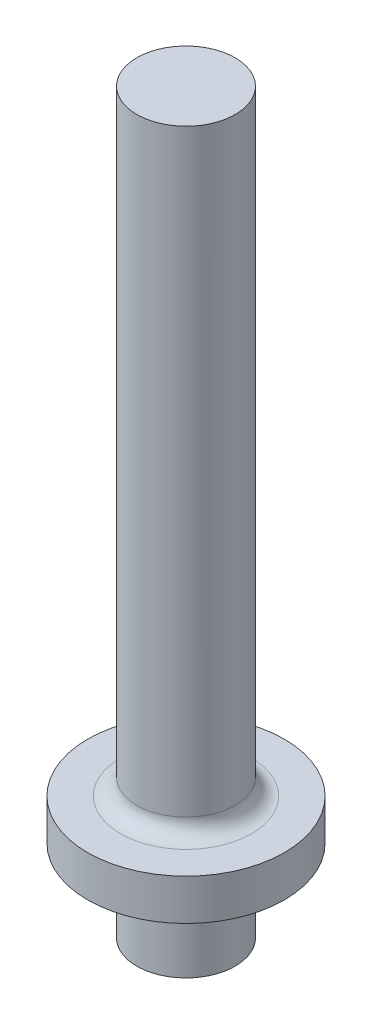
from build123d import *

# Parameters (mm, degrees)
COLLAR_FILLET_R2_R = 2


with BuildPart() as part:
    # Stand Pin Profile → Stand Pin Body (revolve)
    with BuildSketch(Plane.XY, mode=Mode.PRIVATE) as stand_pin_body_sk:
        Polygon((0, 0), (6, 0), (6, 10), (12, 10), (12, 15), (6, 15), (6, 90), (0, 90), align=None)
    revolve(stand_pin_body_sk.sketch.rotate(Axis((0, 90, 0), (0, -1, 0)), 180), axis=Axis((0, 90, 0), (0, -1, 0)))

    # Collar Fillet R2
    collar_fillet_r2_edges = [part.edges().sort_by_distance(p)[0] for p in [
        (6, 15, 0),
    ]]
    fillet(collar_fillet_r2_edges, radius=COLLAR_FILLET_R2_R)


solid = part.part
